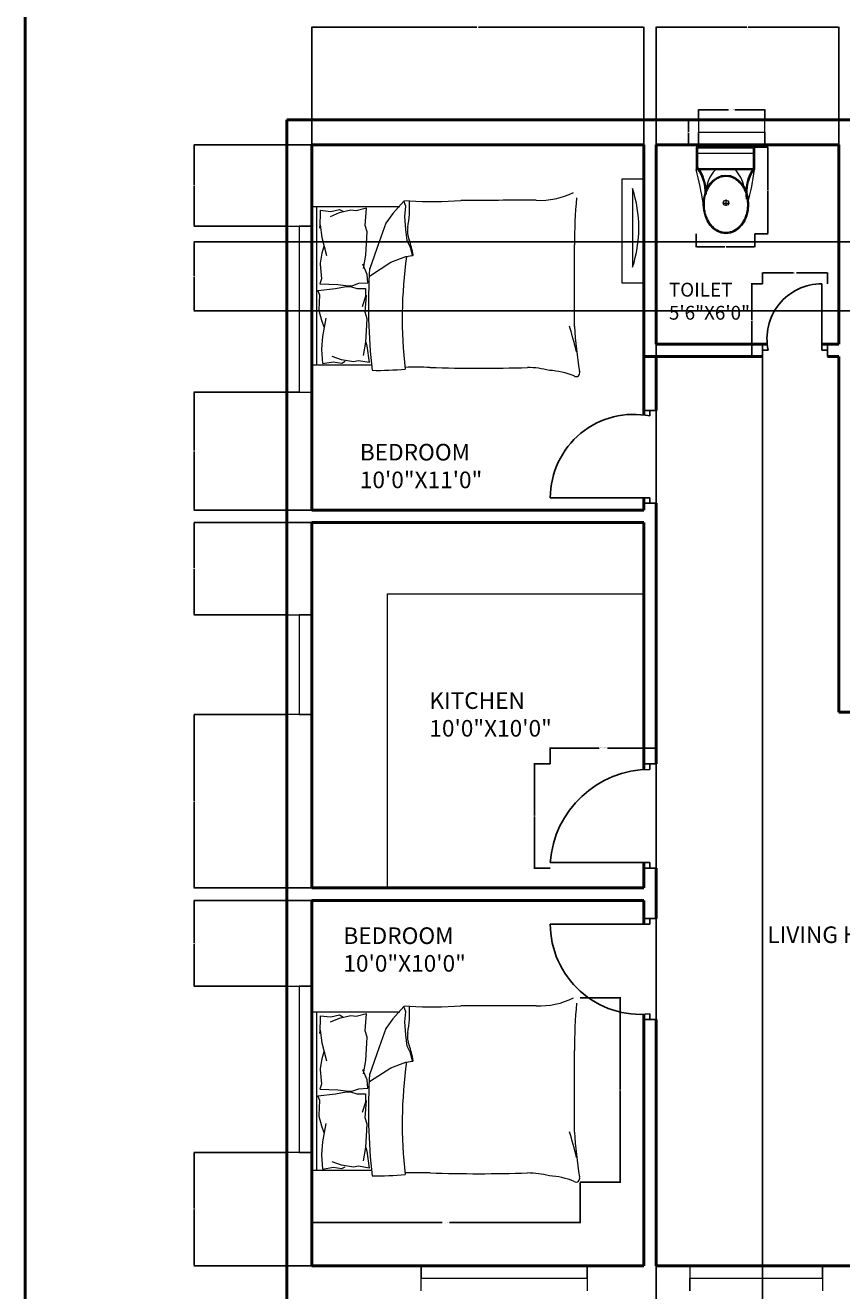
# Model space of a CAD drawing. Units: inches. Extents: x 2268 to 3372, y 1709 to 2892.
# Tile 2 of 6: x 2268 to 2563, y 2040 to 2497. Entities that reach past the tile are written whole.
import ezdxf

# ---------------------------------------------------------------- set-up
doc = ezdxf.new("R2010")
doc.units = ezdxf.units.IN
for name, color, linetype, lineweight in [('A-ANNO-DIMS', 2, 'Continuous', 18), ('A-ANNO-TTLB', 7, 'Continuous', 50), ('A-AREA-IDEN', 7, 'Continuous', 18), ('A-DOOR', 3, 'Continuous', 25), ('A-FLOR-FIXT', 9, 'Continuous', 18), ('A-FURN', 8, 'Continuous', 18), ('A-GLAZ', 4, 'Continuous', 18), ('A-WALL', 7, 'Continuous', 50)]:
    doc.layers.add(name, color=color, linetype=linetype, lineweight=lineweight)
doc.styles.get("Standard").update_dxf_attribs({"font": 'arial.ttf'})
doc.dimstyles.get("Standard").update_dxf_attribs({"dimtxt": 0.18, "dimasz": 0.18, "dimexe": 0.18, "dimexo": 0.0625, "dimgap": 0.09, "dimtad": 0, "dimtih": 1, "dimtoh": 1, "dimdec": 4, "dimzin": 0, "dimdsep": 46, "dimtxsty": 'Standard', "dimcen": 0.09, "dimadec": 0, "dimazin": 0, "dimtfac": 1, "dimtdec": 4, "dimtofl": 0, "dimtmove": 0, "dimatfit": 3, "dimfxl": 1, "dimtolj": 1, "dimtzin": 0, "dimarcsym": 0})

# ---------------------------------------------------------------- blocks, each defined once
blk = doc.blocks.new('A$C31115884')
for p, q in [((283, 498), (223, 498)), ((258, 466), (258, 523)), ((0, 200), (0, 0)), ((520, 200), (0, 200)), ((10, 190), (10, 10)), ((510, 190), (10, 190)), ((510, 10), (510, 190)), ((520, 0), (520, 200)), ((510, 54), (0, 54)), ((10, 10), (510, 10)), ((0, 0), (520, 0))]:
    blk.add_line(p, q)
blk.add_circle((256, 496), 23.6)
for centre, radius, start, end in [((2778, -205), 2807, 165.4549, 171.7133), ((-295, 403), 365, 324.2091, 9.3499), ((-295, 403), 375, 324.2091, 9.3499), ((806, 403), 365, 170.6501, 215.7909), ((3237, 905), 2807, 188.2867, 194.5451), ((384, 406), 293, 190.2774, 224.1564), ((139, 406), 293, 315.8436, 2.6563), ((806, 403), 375, 179.2036, 215.7909)]:
    blk.add_arc(centre, radius, start, end)
blk.add_ellipse((256, 510), major_axis=(0, -261), ratio=0.772727)
blk.add_open_spline([(256, 259), (263, 259), (270, 260), (288, 262), (299, 265), (320, 273), (330, 278), (350, 291), (360, 299), (378, 316), (386, 326), (402, 347), (409, 358), (421, 383), (427, 395), (436, 422), (440, 436), (445, 465), (447, 480), (448, 509), (448, 524), (445, 553), (443, 568), (436, 596), (432, 610), (422, 636), (416, 649), (402, 672), (395, 683), (379, 703), (370, 712), (351, 728), (341, 735), (321, 746), (310, 751), (289, 757), (278, 759), (256, 761), (245, 761), (223, 757), (212, 754), (191, 746), (181, 741), (161, 728), (151, 720), (133, 703), (125, 693), (110, 672), (103, 660), (90, 636), (85, 623), (76, 596), (72, 582), (67, 553), (66, 538), (64, 509), (65, 494), (68, 465), (70, 450), (77, 422), (81, 408), (91, 382), (97, 370), (111, 346), (118, 335), (135, 316), (144, 307), (162, 291), (172, 284), (193, 273), (203, 269), (225, 262), (236, 260), (250, 259), (253, 259), (256, 259)], degree=3, knots=[0, 0, 0, 0, 0.110105, 0.110105, 0.285049, 0.285049, 0.459994, 0.459994, 0.634938, 0.634938, 0.809882, 0.809882, 0.984827, 0.984827, 1.159771, 1.159771, 1.334715, 1.334715, 1.50966, 1.50966, 1.684604, 1.684604, 1.859549, 1.859549, 2.034493, 2.034493, 2.209437, 2.209437, 2.384382, 2.384382, 2.559326, 2.559326, 2.73427, 2.73427, 2.909215, 2.909215, 3.084159, 3.084159, 3.259103, 3.259103, 3.434048, 3.434048, 3.608992, 3.608992, 3.783936, 3.783936, 3.958881, 3.958881, 4.133825, 4.133825, 4.30877, 4.30877, 4.483714, 4.483714, 4.658658, 4.658658, 4.833603, 4.833603, 5.008547, 5.008547, 5.183491, 5.183491, 5.358436, 5.358436, 5.53338, 5.53338, 5.708324, 5.708324, 5.883269, 5.883269, 6.058213, 6.058213, 6.233158, 6.233158, 6.283185, 6.283185, 6.283185, 6.283185])
blk = doc.blocks.new('DOOR-BATH-W')
for p, q in [((21.4, 2.25), (21.4, 26.25)), ((0, 4.5), (0, 0)), ((0, 0), (0, 2.25)), ((0, 2.25), (2, 2.25)), ((23.4, 2.25), (21.4, 2.25)), ((23.4, 4.5), (23.4, 0)), ((23.4, 0), (23.4, 2.25))]:
    blk.add_line(p, q)
blk.add_arc((21.4, 6.41), 19.84, 90, 192.0896)
blk = doc.blocks.new('DOOR-BEDROOM-NW')
for p, q in [((33.75, 33.55), (38.25, 33.55)), ((38.25, 33.55), (36, 33.55)), ((36, 33.55), (36, 31.55)), ((36, 2), (0, 2)), ((33.75, 0), (38.25, 0)), ((36, 0), (36, 2)), ((38.25, 0), (36, 0))]:
    blk.add_line(p, q)
blk.add_arc((30.13, 2), 30.13, 78.7595, 180)
blk = doc.blocks.new('DOOR-BEDROOM-SW')
for p, q in [((36, 34.48), (0, 34.48)), ((33.75, 36.48), (38.25, 36.48)), ((38.25, 36.48), (36, 36.48)), ((36, 36.48), (36, 34.48)), ((33.75, 0), (38.25, 0)), ((36, 0), (36, 2)), ((38.25, 0), (36, 0))]:
    blk.add_line(p, q)
blk.add_arc((32.65, 34.48), 32.65, 180, 275.8823)
blk = doc.blocks.new('DOOR-KITCHEN')
for p, q in [((33.75, 37.66), (38.25, 37.66)), ((38.25, 37.66), (36, 37.66)), ((36, 37.66), (36, 35.66)), ((36, 2), (0, 2)), ((36, 0), (36, 2)), ((33.75, 0), (38.25, 0)), ((38.25, 0), (36, 0))]:
    blk.add_line(p, q)
blk.add_arc((36, -0.42), 36.08, 90, 176.1494)
blk = doc.blocks.new('WIN-48')
for p, q in [((0, 9), (0, 0)), ((48, 4.5), (48, 9)), ((48, 9), (48, 0)), ((0, 0), (0, 4.5)), ((0, 4.5), (48, 4.5))]:
    blk.add_line(p, q)
blk = doc.blocks.new('WIN-60')
for p, q in [((0, 60), (9, 60)), ((9, 60), (4.5, 60)), ((4.5, 60), (4.5, 0)), ((9, 0), (0, 0)), ((4.5, 0), (9, 0))]:
    blk.add_line(p, q)
blk = doc.blocks.new('WIN-60-SPLIT')
for p, q in [((0, 60), (9, 60)), ((9, 60), (4.5, 60)), ((4.5, 60), (4.5, 12)), ((4.5, 12), (4.5, 0)), ((4.5, 0), (0, 0)), ((0, 0), (9, 0))]:
    blk.add_line(p, q)
blk = doc.blocks.new('WIN-36')
for p, q in [((0, 36), (9, 36)), ((9, 36), (4.5, 36)), ((4.5, 36), (4.5, 0)), ((9, 0), (0, 0)), ((4.5, 0), (9, 0))]:
    blk.add_line(p, q)
blk = doc.blocks.new('WIN-24-TRANSVERSE')
for p, q in [((0, 9), (0, 0)), ((24, 0), (24, 9)), ((0, 0), (0, 4.5)), ((0, 4.5), (24, 4.5)), ((24, 4.5), (24, 0))]:
    blk.add_line(p, q)
blk = doc.blocks.new('COUNTER-KITCHEN-L')
for p, q in [((0, 0), (0, 106.22)), ((0, 106.22), (92.56, 106.22))]:
    blk.add_line(p, q)
blk = doc.blocks.new('BEDROOM-WALL-UNIT')
blk.add_line((3.85, 34.02), (3.85, 5.6))
blk.add_lwpolyline([(7.87, 37.37), (0, 37.37), (0, 0), (7.87, 0)], close=True)
blk.add_arc((-39.98, 19.81), 46.08, 342.0375, 17.9625)
blk = doc.blocks.new('BED-DOUBLE')
for p, q in [((0, 61.46), (31.9, 61.46)), ((0, 4.17), (0, 61.46)), ((1.84, 4.17), (1.84, 61.46)), ((3.07, 60.08), (2.95, 53.6)), ((3.07, 60.08), (6.92, 59.62)), ((6.92, 59.62), (10, 60.34)), ((14.18, 60.08), (9.9, 59.11)), ((10, 60.34), (11.25, 59.72)), ((16.11, 59.85), (14.18, 60.08)), ((19.87, 60.78), (16.11, 59.85)), ((19.38, 54.63), (19.87, 60.78)), ((33.26, 63.38), (29.37, 58.94)), ((35.36, 63.48), (33.26, 63.38, 4.64)), ((34.01, 61.54), (33.26, 63.38)), ((33.63, 57.82), (34.01, 61.54)), ((9.9, 59.11), (6.69, 57.7)), ((26.77, 55.41), (24.36, 48.73)), ((29.37, 58.94), (26.77, 55.41)), ((34.01, 53.18), (33.63, 57.82)), ((2.95, 53.6), (3.05, 54.8)), ((3.05, 54.8), (3.68, 50.25)), ((20.05, 52.28), (19.38, 54.63)), ((19.54, 43.87), (20.05, 52.28)), ((34.56, 49.1), (34.01, 53.18)), ((3.68, 50.25), (5.3, 43.75)), ((4.4, 47), (3.69, 44.52)), ((24.36, 48.73), (20.84, 38.73)), ((35.68, 46.68), (34.56, 49.1)), ((36.42, 43.71), (35.68, 46.68)), ((95, 18.06), (95, 47.57)), ((3.69, 44.52), (3.04, 41.01)), ((18.74, 39.04), (19.54, 43.87)), ((20.84, 36.28), (28.62, 41.3)), ((28.62, 41.3), (34.01, 43.34)), ((34.01, 43.34), (36.42, 43.71)), ((3.04, 41.01), (3.07, 40.62)), ((3.07, 40.62), (3.57, 35.31)), ((20.07, 36.86), (18.53, 40.55)), ((20.25, 33.92), (20.07, 36.86)), ((3.57, 35.31), (2.99, 33.54)), ((2.99, 33.54), (9.43, 33.25)), ((8.66, 31.84), (12.47, 32.54)), ((9.43, 33.25), (13.28, 32.79)), ((12.47, 32.54), (14.03, 32.54)), ((13.28, 32.79), (14.84, 32.89)), ((14.03, 32.54), (16.28, 31.84)), ((14.84, 32.89), (17.04, 33.72)), ((17.04, 33.72), (20.25, 33.92)), ((2.24, 31.15), (8.66, 31.84)), ((2.94, 29.42), (2.24, 31.15)), ((2.76, 24.09), (2.94, 29.42)), ((16.28, 31.84), (19.5, 31.84)), ((19.5, 28.9), (18.19, 25.13)), ((19.38, 23.24), (19.87, 29.39)), ((19.5, 31.84), (19.5, 28.9)), ((2.76, 23.7), (2.76, 24.09)), ((3.63, 20.23), (2.76, 23.7)), ((20.05, 20.89), (19.38, 23.24)), ((4.5, 17.81), (3.63, 20.23)), ((3.98, 14.52), (5.19, 21.1)), ((19.54, 12.48), (20.05, 20.89)), ((3.63, 9.93), (3.98, 14.52)), ((3.61, 9.81), (3.63, 9.93)), ((4, 4.67), (3.61, 9.81)), ((18.74, 7.65), (19.54, 12.48)), ((19.54, 12.48), (19.92, 11.13)), ((19.92, 11.13), (20.79, 5.02)), ((3.98, 4.67), (7.79, 5.36)), ((10.74, 6.06), (7.44, 7.27)), ((7.79, 5.36), (10.91, 4.84)), ((15.07, 5.36), (10.74, 6.06)), ((10.91, 4.84), (12.12, 5.54)), ((16.98, 5.71), (15.07, 5.36)), ((20.79, 5.02), (16.98, 5.71)), ((21.71, 4.17), (0, 4.17))]:
    blk.add_line(p, q)
for centre, radius, start, end in [((82.32, 91.3), 27.65, 267.4714, 296.4681), ((254.49, 49.33), 159.5, 174.4998, 180.6351), ((-7.98, 61.53), 43.38, 349.8763, 2.5657), ((43.54, 218.51), 155.25, 266.9791, 273.8365), ((81.31, -5405.34), 5469.02, 90.00217, 90.28689), ((42.04, 52.44), 7.46, 168.6608, 203.7384), ((1.78, 37.35), 35.55, 10.6617, 19.8806), ((187.4, 21.29), 154.68, 171.7845, 186.9006), ((36.49, 43.92), 0.221, 250.2464, 1.1377), ((218.26, 25.61), 197.77, 176.0865, 186.7821), ((-28.43, -20.65), 127.63, 13.3832, 17.7053), ((240.78, 25.69), 145.97, 182.9958, 189.4091), ((24.09, 102.1), 99.87, 268.7218, 275.604), ((37.37, -200.58), 203.94, 88.4762, 91.0082), ((60.68, 581.23), 578.22, 268.22771, 271.71854), ((77.34, -32.25), 35.53, 76.0648, 88.9113), ((84.25, -25.97), 28.25, 67.9751, 86.652), ((95.57, 1.3), 1.31, 236.1736, 23.4781)]:
    blk.add_arc(centre, radius, start, end)
blk = doc.blocks.new('*D34')
at = {"layer": 'A-ANNO-DIMS', "color": 0, "lineweight": -2, "transparency": 16777216}
for p, q in [((2534.82, 2403.93), (2530.76, 2403.93)), ((2530.94, 2403.75), (2530.94, 2390.98)), ((2530.94, 2377.86), (2530.94, 2390.62)), ((2534.82, 2377.68), (2530.76, 2377.68))]:
    blk.add_line(p, q, dxfattribs=at)
at = {"layer": 'A-ANNO-DIMS', "color": 0, "transparency": 16777216}
for points in [[(2530.91, 2403.75), (2530.97, 2403.75), (2530.94, 2403.93)], [(2530.91, 2377.86), (2530.97, 2377.86), (2530.94, 2377.68)]]:
    blk.add_solid(points, dxfattribs=at)
at = {"layer": 'Defpoints', "color": 0, "transparency": 16777216}
for p in [(2530.94, 2403.93), (2534.88, 2403.93), (2534.88, 2377.68)]:
    blk.add_point(p, dxfattribs=at)
at = {"layer": 'A-ANNO-DIMS', "color": 0, "transparency": 16777216, "insert": (2530.94, 2390.8), "char_height": 0.18, "attachment_point": 5}
blk.add_mtext('\\A1;DOOR 26 TYP.', dxfattribs=at)
blk = doc.blocks.new('*D35')
at = {"layer": 'A-ANNO-DIMS', "color": 0, "lineweight": -2, "transparency": 16777216}
for p, q in [((2534.88, 2403.99), (2534.88, 2408.04)), ((2535.06, 2407.86), (2546.05, 2407.86)), ((2558.1, 2407.86), (2547.11, 2407.86)), ((2558.28, 2403.99), (2558.28, 2408.04))]:
    blk.add_line(p, q, dxfattribs=at)
at = {"layer": 'A-ANNO-DIMS', "color": 0, "transparency": 16777216}
for points in [[(2535.06, 2407.89), (2535.06, 2407.83), (2534.88, 2407.86)], [(2558.1, 2407.89), (2558.1, 2407.83), (2558.28, 2407.86)]]:
    blk.add_solid(points, dxfattribs=at)
at = {"layer": 'Defpoints', "color": 0, "transparency": 16777216}
for p in [(2558.28, 2407.86), (2534.88, 2403.93), (2558.28, 2403.93)]:
    blk.add_point(p, dxfattribs=at)
at = {"layer": 'A-ANNO-DIMS', "color": 0, "transparency": 16777216, "insert": (2546.58, 2407.86), "char_height": 0.18, "attachment_point": 5}
blk.add_mtext('\\A1;23 TYP.', dxfattribs=at)
blk = doc.blocks.new('*D42')
at = {"layer": 'A-ANNO-DIMS', "color": 0, "lineweight": -2, "transparency": 16777216}
for p, q in [((2458.14, 2230.55), (2458.14, 2236.4)), ((2458.32, 2236.22), (2475.75, 2236.22)), ((2496.21, 2236.22), (2478.79, 2236.22)), ((2496.39, 2230.55), (2496.39, 2236.4))]:
    blk.add_line(p, q, dxfattribs=at)
at = {"layer": 'A-ANNO-DIMS', "color": 0, "transparency": 16777216}
for points in [[(2458.32, 2236.25), (2458.32, 2236.19), (2458.14, 2236.22)], [(2496.21, 2236.25), (2496.21, 2236.19), (2496.39, 2236.22)]]:
    blk.add_solid(points, dxfattribs=at)
at = {"layer": 'Defpoints', "color": 0, "transparency": 16777216}
for p in [(2496.39, 2236.22), (2458.14, 2230.49), (2496.39, 2230.49)]:
    blk.add_point(p, dxfattribs=at)
at = {"layer": 'A-ANNO-DIMS', "color": 0, "transparency": 16777216, "insert": (2477.27, 2236.22), "char_height": 0.18, "attachment_point": 5}
blk.add_mtext('\\A1;KITCHEN DOOR 38 TYP.', dxfattribs=at)
blk = doc.blocks.new('*D43')
at = {"layer": 'A-ANNO-DIMS', "color": 0, "lineweight": -2, "transparency": 16777216}
for p, q in [((2458.08, 2230.49), (2452.23, 2230.49)), ((2452.41, 2230.31), (2452.41, 2211.84)), ((2452.41, 2193.01), (2452.41, 2211.47)), ((2458.08, 2192.83), (2452.23, 2192.83))]:
    blk.add_line(p, q, dxfattribs=at)
at = {"layer": 'A-ANNO-DIMS', "color": 0, "transparency": 16777216}
for points in [[(2452.38, 2230.31), (2452.44, 2230.31), (2452.41, 2230.49)], [(2452.38, 2193.01), (2452.44, 2193.01), (2452.41, 2192.83)]]:
    blk.add_solid(points, dxfattribs=at)
at = {"layer": 'Defpoints', "color": 0, "transparency": 16777216}
for p in [(2452.41, 2230.49), (2458.14, 2230.49), (2458.14, 2192.83)]:
    blk.add_point(p, dxfattribs=at)
at = {"layer": 'A-ANNO-DIMS', "color": 0, "transparency": 16777216, "insert": (2452.41, 2211.66), "char_height": 0.18, "attachment_point": 5}
blk.add_mtext('\\A1;38 TYP.', dxfattribs=at)
blk = doc.blocks.new('*D48')
at = {"layer": 'A-ANNO-DIMS', "color": 0, "lineweight": -2, "transparency": 16777216}
for p, q in [((2511.69, 2463.24), (2511.69, 2466.96)), ((2511.87, 2466.78), (2522.57, 2466.78)), ((2535.51, 2466.78), (2524.81, 2466.78)), ((2535.69, 2463.24), (2535.69, 2466.96))]:
    blk.add_line(p, q, dxfattribs=at)
at = {"layer": 'A-ANNO-DIMS', "color": 0, "transparency": 16777216}
for points in [[(2511.87, 2466.81), (2511.87, 2466.75), (2511.69, 2466.78)], [(2535.51, 2466.81), (2535.51, 2466.75), (2535.69, 2466.78)]]:
    blk.add_solid(points, dxfattribs=at)
at = {"layer": 'Defpoints', "color": 0, "transparency": 16777216}
for p in [(2535.69, 2466.78), (2511.69, 2463.18), (2535.69, 2463.18)]:
    blk.add_point(p, dxfattribs=at)
at = {"layer": 'A-ANNO-DIMS', "color": 0, "transparency": 16777216, "insert": (2523.69, 2466.78), "char_height": 0.18, "attachment_point": 5}
blk.add_mtext('\\A1;WINDOW 24 TYP.', dxfattribs=at)
blk = doc.blocks.new('*D49')
at = {"layer": 'A-ANNO-DIMS', "color": 0, "lineweight": -2, "transparency": 16777216}
for p, q in [((2511.63, 2463.18), (2507.91, 2463.18)), ((2508.09, 2463), (2508.09, 2458.86)), ((2508.09, 2454.36), (2508.09, 2458.49)), ((2511.63, 2454.18), (2507.91, 2454.18))]:
    blk.add_line(p, q, dxfattribs=at)
at = {"layer": 'A-ANNO-DIMS', "color": 0, "transparency": 16777216}
for points in [[(2508.06, 2463), (2508.12, 2463), (2508.09, 2463.18)], [(2508.06, 2454.36), (2508.12, 2454.36), (2508.09, 2454.18)]]:
    blk.add_solid(points, dxfattribs=at)
at = {"layer": 'Defpoints', "color": 0, "transparency": 16777216}
for p in [(2508.09, 2463.18), (2511.69, 2463.18), (2511.69, 2454.18)]:
    blk.add_point(p, dxfattribs=at)
at = {"layer": 'A-ANNO-DIMS', "color": 0, "transparency": 16777216, "insert": (2508.09, 2458.68), "char_height": 0.18, "attachment_point": 5}
blk.add_mtext('\\A1;9 TYP.', dxfattribs=at)
blk = doc.blocks.new('*D70')
at = {"layer": 'A-ANNO-DIMS', "color": 0, "lineweight": -2, "transparency": 16777216}
for p, q in [((2371.89, 2079.27), (2371.89, 2064.61)), ((2468.89, 2079.27), (2468.89, 2064.61)), ((2372.07, 2064.79), (2419.02, 2064.79)), ((2468.71, 2064.79), (2421.76, 2064.79))]:
    blk.add_line(p, q, dxfattribs=at)
at = {"layer": 'A-ANNO-DIMS', "color": 0, "transparency": 16777216}
for points in [[(2372.07, 2064.82), (2372.07, 2064.76), (2371.89, 2064.79)], [(2468.71, 2064.82), (2468.71, 2064.76), (2468.89, 2064.79)]]:
    blk.add_solid(points, dxfattribs=at)
at = {"layer": 'Defpoints', "color": 0, "transparency": 16777216}
for p in [(2371.89, 2079.34), (2468.89, 2079.34), (2468.89, 2064.79)]:
    blk.add_point(p, dxfattribs=at)
at = {"layer": 'A-ANNO-DIMS', "color": 0, "transparency": 16777216, "insert": (2420.39, 2064.79), "char_height": 0.18, "attachment_point": 5}
blk.add_mtext('\\A1;DOUBLE BED 97 TYP.', dxfattribs=at)
blk = doc.blocks.new('*D71')
at = {"layer": 'A-ANNO-DIMS', "color": 0, "lineweight": -2, "transparency": 16777216}
for p, q in [((2468.96, 2145.99), (2483.62, 2145.99)), ((2483.44, 2145.81), (2483.44, 2112.84)), ((2483.44, 2079.52), (2483.44, 2112.48)), ((2468.96, 2079.34), (2483.62, 2079.34))]:
    blk.add_line(p, q, dxfattribs=at)
at = {"layer": 'A-ANNO-DIMS', "color": 0, "transparency": 16777216}
for points in [[(2483.41, 2145.81), (2483.47, 2145.81), (2483.44, 2145.99)], [(2483.41, 2079.52), (2483.47, 2079.52), (2483.44, 2079.34)]]:
    blk.add_solid(points, dxfattribs=at)
at = {"layer": 'Defpoints', "color": 0, "transparency": 16777216}
for p in [(2468.89, 2145.99), (2483.44, 2145.99), (2468.89, 2079.34)]:
    blk.add_point(p, dxfattribs=at)
at = {"layer": 'A-ANNO-DIMS', "color": 0, "transparency": 16777216, "insert": (2483.44, 2112.66), "char_height": 0.18, "attachment_point": 5}
blk.add_mtext('\\A1;67 TYP.', dxfattribs=at)
blk = doc.blocks.new('*D74')
at = {"layer": 'A-ANNO-DIMS', "color": 0, "lineweight": -2, "transparency": 16777216}
for p, q in [((2532.07, 2453.35), (2536.88, 2453.35)), ((2536.7, 2453.17), (2536.7, 2437.88)), ((2536.7, 2422.22), (2536.7, 2437.51)), ((2532.07, 2422.04), (2536.88, 2422.04))]:
    blk.add_line(p, q, dxfattribs=at)
at = {"layer": 'A-ANNO-DIMS', "color": 0, "transparency": 16777216}
for points in [[(2536.67, 2453.17), (2536.73, 2453.17), (2536.7, 2453.35)], [(2536.67, 2422.22), (2536.73, 2422.22), (2536.7, 2422.04)]]:
    blk.add_solid(points, dxfattribs=at)
at = {"layer": 'Defpoints', "color": 0, "transparency": 16777216}
for p in [(2532, 2453.35), (2532, 2422.04), (2536.7, 2422.04)]:
    blk.add_point(p, dxfattribs=at)
at = {"layer": 'A-ANNO-DIMS', "color": 0, "transparency": 16777216, "insert": (2536.7, 2437.7), "char_height": 0.18, "attachment_point": 5}
blk.add_mtext('\\A1;WC 31', dxfattribs=at)
blk = doc.blocks.new('*D75')
at = {"layer": 'A-ANNO-DIMS', "color": 0, "lineweight": -2, "transparency": 16777216}
for p, q in [((2510.88, 2421.98), (2510.88, 2417.17)), ((2532, 2421.98), (2532, 2417.17)), ((2511.06, 2417.35), (2521.24, 2417.35)), ((2531.82, 2417.35), (2521.65, 2417.35))]:
    blk.add_line(p, q, dxfattribs=at)
at = {"layer": 'A-ANNO-DIMS', "color": 0, "transparency": 16777216}
for points in [[(2511.06, 2417.38), (2511.06, 2417.32), (2510.88, 2417.35)], [(2531.82, 2417.38), (2531.82, 2417.32), (2532, 2417.35)]]:
    blk.add_solid(points, dxfattribs=at)
at = {"layer": 'Defpoints', "color": 0, "transparency": 16777216}
for p in [(2510.88, 2422.04), (2532, 2422.04), (2510.88, 2417.35)]:
    blk.add_point(p, dxfattribs=at)
at = {"layer": 'A-ANNO-DIMS', "color": 0, "transparency": 16777216, "insert": (2521.44, 2417.35), "char_height": 0.18, "attachment_point": 5}
blk.add_mtext('\\A1;21', dxfattribs=at)
blk = doc.blocks.new('*D78')
at = {"layer": 'A-ANNO-DIMS', "color": 0, "lineweight": -2, "transparency": 16777216}
for p, q in [((2371.89, 2454.24), (2371.89, 2496.81)), ((2372.07, 2496.63), (2431.61, 2496.63)), ((2491.71, 2496.63), (2432.17, 2496.63)), ((2491.89, 2454.24), (2491.89, 2496.81))]:
    blk.add_line(p, q, dxfattribs=at)
at = {"layer": 'A-ANNO-DIMS', "color": 0, "transparency": 16777216}
for points in [[(2372.07, 2496.66), (2372.07, 2496.6), (2371.89, 2496.63)], [(2491.71, 2496.66), (2491.71, 2496.6), (2491.89, 2496.63)]]:
    blk.add_solid(points, dxfattribs=at)
at = {"layer": 'Defpoints', "color": 0, "transparency": 16777216}
for p in [(2491.89, 2496.63), (2371.89, 2454.18), (2491.89, 2454.18)]:
    blk.add_point(p, dxfattribs=at)
at = {"layer": 'A-ANNO-DIMS', "color": 0, "transparency": 16777216, "insert": (2431.89, 2496.63), "char_height": 0.18, "attachment_point": 5}
blk.add_mtext('\\A1;120', dxfattribs=at)
blk = doc.blocks.new('*D79')
at = {"layer": 'A-ANNO-DIMS', "color": 0, "lineweight": -2, "transparency": 16777216}
for p, q in [((2496.39, 2454.24), (2496.39, 2496.81)), ((2496.57, 2496.63), (2529.17, 2496.63)), ((2562.21, 2496.63), (2529.61, 2496.63)), ((2562.39, 2454.24), (2562.39, 2496.81))]:
    blk.add_line(p, q, dxfattribs=at)
at = {"layer": 'A-ANNO-DIMS', "color": 0, "transparency": 16777216}
for points in [[(2496.57, 2496.66), (2496.57, 2496.6), (2496.39, 2496.63)], [(2562.21, 2496.66), (2562.21, 2496.6), (2562.39, 2496.63)]]:
    blk.add_solid(points, dxfattribs=at)
at = {"layer": 'Defpoints', "color": 0, "transparency": 16777216}
for p in [(2562.39, 2496.63), (2496.39, 2454.18), (2562.39, 2454.18)]:
    blk.add_point(p, dxfattribs=at)
at = {"layer": 'A-ANNO-DIMS', "color": 0, "transparency": 16777216, "insert": (2529.39, 2496.63), "char_height": 0.18, "attachment_point": 5}
blk.add_mtext('\\A1;66', dxfattribs=at)
blk = doc.blocks.new('*D81')
at = {"layer": 'A-ANNO-DIMS', "color": 0, "lineweight": -2, "transparency": 16777216}
for p, q in [((2496.39, 2382.11), (2496.39, 1790.27)), ((2534.88, 2377.61), (2534.88, 1790.27)), ((2496.57, 1790.45), (2515.17, 1790.45)), ((2534.7, 1790.45), (2516.1, 1790.45))]:
    blk.add_line(p, q, dxfattribs=at)
at = {"layer": 'A-ANNO-DIMS', "color": 0, "transparency": 16777216}
for points in [[(2496.57, 1790.48), (2496.57, 1790.42), (2496.39, 1790.45)], [(2534.7, 1790.48), (2534.7, 1790.42), (2534.88, 1790.45)]]:
    blk.add_solid(points, dxfattribs=at)
at = {"layer": 'Defpoints', "color": 0, "transparency": 16777216}
for p in [(2496.39, 2382.18), (2534.88, 2377.68), (2534.88, 1790.45)]:
    blk.add_point(p, dxfattribs=at)
at = {"layer": 'A-ANNO-DIMS', "color": 0, "transparency": 16777216, "insert": (2515.64, 1790.45), "char_height": 0.18, "attachment_point": 5}
blk.add_mtext('\\A1;38.486', dxfattribs=at)
blk = doc.blocks.new('*D84')
at = {"layer": 'A-ANNO-DIMS', "color": 0, "lineweight": -2, "transparency": 16777216}
for p, q in [((2362.83, 2090.16), (2329.26, 2090.16)), ((2329.44, 2089.98), (2329.44, 2069.85)), ((2329.44, 2049.36), (2329.44, 2069.49)), ((2371.83, 2049.18), (2329.26, 2049.18))]:
    blk.add_line(p, q, dxfattribs=at)
at = {"layer": 'A-ANNO-DIMS', "color": 0, "transparency": 16777216}
for points in [[(2329.41, 2089.98), (2329.47, 2089.98), (2329.44, 2090.16)], [(2329.41, 2049.36), (2329.47, 2049.36), (2329.44, 2049.18)]]:
    blk.add_solid(points, dxfattribs=at)
at = {"layer": 'Defpoints', "color": 0, "transparency": 16777216}
for p in [(2329.44, 2090.16), (2362.89, 2090.16), (2371.89, 2049.18)]:
    blk.add_point(p, dxfattribs=at)
at = {"layer": 'A-ANNO-DIMS', "color": 0, "transparency": 16777216, "insert": (2329.44, 2069.67), "char_height": 0.18, "attachment_point": 5}
blk.add_mtext('\\A1;40.986', dxfattribs=at)
blk = doc.blocks.new('*D85')
at = {"layer": 'A-ANNO-DIMS', "color": 0, "lineweight": -2, "transparency": 16777216}
for p, q in [((2371.83, 2181.18), (2329.26, 2181.18)), ((2329.44, 2181), (2329.44, 2165.85)), ((2329.44, 2150.34), (2329.44, 2165.49)), ((2362.83, 2150.16), (2329.26, 2150.16))]:
    blk.add_line(p, q, dxfattribs=at)
at = {"layer": 'A-ANNO-DIMS', "color": 0, "transparency": 16777216}
for points in [[(2329.41, 2181), (2329.47, 2181), (2329.44, 2181.18)], [(2329.41, 2150.34), (2329.47, 2150.34), (2329.44, 2150.16)]]:
    blk.add_solid(points, dxfattribs=at)
at = {"layer": 'Defpoints', "color": 0, "transparency": 16777216}
for p in [(2329.44, 2181.18), (2371.89, 2181.18), (2362.89, 2150.16)]:
    blk.add_point(p, dxfattribs=at)
at = {"layer": 'A-ANNO-DIMS', "color": 0, "transparency": 16777216, "insert": (2329.44, 2165.67), "char_height": 0.18, "attachment_point": 5}
blk.add_mtext('\\A1;31.014', dxfattribs=at)
blk = doc.blocks.new('*D86')
at = {"layer": 'A-ANNO-DIMS', "color": 0, "lineweight": -2, "transparency": 16777216}
for p, q in [((2362.83, 2248.31), (2329.26, 2248.31)), ((2329.44, 2248.13), (2329.44, 2217.17)), ((2329.44, 2185.86), (2329.44, 2216.81)), ((2371.83, 2185.68), (2329.26, 2185.68))]:
    blk.add_line(p, q, dxfattribs=at)
at = {"layer": 'A-ANNO-DIMS', "color": 0, "transparency": 16777216}
for points in [[(2329.41, 2248.13), (2329.47, 2248.13), (2329.44, 2248.31)], [(2329.41, 2185.86), (2329.47, 2185.86), (2329.44, 2185.68)]]:
    blk.add_solid(points, dxfattribs=at)
at = {"layer": 'Defpoints', "color": 0, "transparency": 16777216}
for p in [(2329.44, 2248.31), (2362.89, 2248.31), (2371.89, 2185.68)]:
    blk.add_point(p, dxfattribs=at)
at = {"layer": 'A-ANNO-DIMS', "color": 0, "transparency": 16777216, "insert": (2329.44, 2216.99), "char_height": 0.18, "attachment_point": 5}
blk.add_mtext('\\A1;62.63', dxfattribs=at)
blk = doc.blocks.new('*D87')
at = {"layer": 'A-ANNO-DIMS', "color": 0, "lineweight": -2, "transparency": 16777216}
for p, q in [((2371.83, 2317.68), (2329.26, 2317.68)), ((2329.44, 2317.5), (2329.44, 2301.17)), ((2329.44, 2284.49), (2329.44, 2300.81)), ((2362.83, 2284.31), (2329.26, 2284.31))]:
    blk.add_line(p, q, dxfattribs=at)
at = {"layer": 'A-ANNO-DIMS', "color": 0, "transparency": 16777216}
for points in [[(2329.41, 2317.5), (2329.47, 2317.5), (2329.44, 2317.68)], [(2329.41, 2284.49), (2329.47, 2284.49), (2329.44, 2284.31)]]:
    blk.add_solid(points, dxfattribs=at)
at = {"layer": 'Defpoints', "color": 0, "transparency": 16777216}
for p in [(2329.44, 2317.68), (2371.89, 2317.68), (2362.89, 2284.31)]:
    blk.add_point(p, dxfattribs=at)
at = {"layer": 'A-ANNO-DIMS', "color": 0, "transparency": 16777216, "insert": (2329.44, 2300.99), "char_height": 0.18, "attachment_point": 5}
blk.add_mtext('\\A1;33.37', dxfattribs=at)
blk = doc.blocks.new('*D88')
at = {"layer": 'A-ANNO-DIMS', "color": 0, "lineweight": -2, "transparency": 16777216}
for p, q in [((2362.83, 2364.81), (2329.26, 2364.81)), ((2329.44, 2364.63), (2329.44, 2343.68)), ((2329.44, 2322.36), (2329.44, 2343.31)), ((2371.83, 2322.18), (2329.26, 2322.18))]:
    blk.add_line(p, q, dxfattribs=at)
at = {"layer": 'A-ANNO-DIMS', "color": 0, "transparency": 16777216}
for points in [[(2329.41, 2364.63), (2329.47, 2364.63), (2329.44, 2364.81)], [(2329.41, 2322.36), (2329.47, 2322.36), (2329.44, 2322.18)]]:
    blk.add_solid(points, dxfattribs=at)
at = {"layer": 'Defpoints', "color": 0, "transparency": 16777216}
for p in [(2329.44, 2364.81), (2362.89, 2364.81), (2371.89, 2322.18)]:
    blk.add_point(p, dxfattribs=at)
at = {"layer": 'A-ANNO-DIMS', "color": 0, "transparency": 16777216, "insert": (2329.44, 2343.49), "char_height": 0.18, "attachment_point": 5}
blk.add_mtext('\\A1;42.64', dxfattribs=at)
blk = doc.blocks.new('*D89')
at = {"layer": 'A-ANNO-DIMS', "color": 0, "lineweight": -2, "transparency": 16777216}
for p, q in [((2371.83, 2454.18), (2329.26, 2454.18)), ((2329.44, 2454), (2329.44, 2439.68)), ((2329.44, 2424.99), (2329.44, 2439.31)), ((2362.83, 2424.81), (2329.26, 2424.81))]:
    blk.add_line(p, q, dxfattribs=at)
at = {"layer": 'A-ANNO-DIMS', "color": 0, "transparency": 16777216}
for points in [[(2329.41, 2454), (2329.47, 2454), (2329.44, 2454.18)], [(2329.41, 2424.99), (2329.47, 2424.99), (2329.44, 2424.81)]]:
    blk.add_solid(points, dxfattribs=at)
at = {"layer": 'Defpoints', "color": 0, "transparency": 16777216}
for p in [(2329.44, 2454.18), (2371.89, 2454.18), (2362.89, 2424.81)]:
    blk.add_point(p, dxfattribs=at)
at = {"layer": 'A-ANNO-DIMS', "color": 0, "transparency": 16777216, "insert": (2329.44, 2439.49), "char_height": 0.18, "attachment_point": 5}
blk.add_mtext('\\A1;29.36', dxfattribs=at)
blk = doc.blocks.new('*D98')
at = {"layer": 'A-ANNO-DIMS', "color": 0, "lineweight": -2, "transparency": 16777216}
for p, q in [((2703.83, 2419.05), (2329.26, 2419.05)), ((2329.44, 2418.87), (2329.44, 2406.8)), ((2329.44, 2394.36), (2329.44, 2406.43)), ((2703.83, 2394.18), (2329.26, 2394.18))]:
    blk.add_line(p, q, dxfattribs=at)
at = {"layer": 'A-ANNO-DIMS', "color": 0, "transparency": 16777216}
for points in [[(2329.41, 2418.87), (2329.47, 2418.87), (2329.44, 2419.05)], [(2329.41, 2394.36), (2329.47, 2394.36), (2329.44, 2394.18)]]:
    blk.add_solid(points, dxfattribs=at)
at = {"layer": 'Defpoints', "color": 0, "transparency": 16777216}
for p in [(2329.44, 2419.05), (2703.89, 2419.05), (2703.89, 2394.18)]:
    blk.add_point(p, dxfattribs=at)
at = {"layer": 'A-ANNO-DIMS', "color": 0, "transparency": 16777216, "insert": (2329.44, 2406.61), "char_height": 0.18, "attachment_point": 5}
blk.add_mtext('\\A1;24.88', dxfattribs=at)

msp = doc.modelspace()

# ---------------------------------------------------------------- linework, layer by layer
at = {"layer": 'A-ANNO-TTLB'}
msp.add_lwpolyline([(2268.3884, 2892.2471), (3372.3464, 2892.2471), (3372.3464, 1709.0755), (2268.3884, 1709.0755)], close=True, dxfattribs=at)
at = {"layer": 'A-WALL'}
for p, q in [((2362.8943, 2463.1756), (2712.8943, 2463.1756)), ((2362.8943, 2463.1756), (2712.8943, 2463.1756)), ((2362.8943, 2463.1756), (2362.8943, 1877.1756)), ((2362.8943, 2463.1756), (2712.8943, 2463.1756)), ((2362.8943, 2463.1756), (2712.8943, 2463.1756)), ((2362.8943, 2463.1756), (2362.8943, 1877.1756)), ((2371.8943, 2454.1756), (2491.8943, 2454.1756)), ((2371.8943, 2454.1756), (2371.8943, 2322.1756)), ((2371.8943, 2454.1756), (2491.8943, 2454.1756)), ((2371.8943, 2454.1756), (2371.8943, 2322.1756)), ((2491.8943, 2454.1756), (2491.8943, 2356.5449)), ((2491.8943, 2454.1756), (2491.8943, 2356.5449)), ((2496.3943, 2454.1756), (2496.3943, 2382.1756)), ((2496.3943, 2454.1756), (2562.3943, 2454.1756)), ((2496.3943, 2454.1756), (2562.3943, 2454.1756)), ((2496.3943, 2454.1756), (2496.3943, 2382.1756)), ((2562.3943, 2454.1756), (2562.3943, 2382.1756)), ((2562.3943, 2454.1756), (2562.3943, 2382.1756)), ((2496.3943, 2382.1756), (2536.5315, 2382.1756)), ((2496.3943, 2382.1756), (2536.5315, 2382.1756)), ((2556.2836, 2382.1756), (2562.3943, 2382.1756)), ((2556.2836, 2382.1756), (2562.3943, 2382.1756)), ((2491.8943, 2377.6756), (2534.8799, 2377.6756)), ((2491.8943, 2377.6756), (2534.8799, 2377.6756)), ((2496.3943, 2377.6756), (2496.3943, 2358.1856)), ((2496.3943, 2377.6756), (2496.3943, 2358.1856)), ((2558.2836, 2377.6756), (2562.3943, 2377.6756)), ((2558.2836, 2377.6756), (2562.3943, 2377.6756)), ((2562.3943, 2377.6756), (2562.3943, 2249.1756)), ((2562.3943, 2377.6756), (2562.3943, 2249.1756)), ((2491.8943, 2326.6361), (2491.8943, 2322.1756)), ((2491.8943, 2326.6361), (2491.8943, 2322.1756)), ((2496.3943, 2324.6361), (2496.3943, 2230.4862)), ((2496.3943, 2324.6361), (2496.3943, 2230.4862)), ((2371.8943, 2322.1756), (2491.8943, 2322.1756)), ((2371.8943, 2322.1756), (2491.8943, 2322.1756)), ((2371.8943, 2317.6756), (2491.8943, 2317.6756)), ((2371.8943, 2317.6756), (2371.8943, 2185.6756)), ((2371.8943, 2317.6756), (2491.8943, 2317.6756)), ((2371.8943, 2317.6756), (2371.8943, 2185.6756)), ((2491.8943, 2317.6756), (2491.8943, 2228.4159)), ((2491.8943, 2317.6756), (2491.8943, 2228.4159)), ((2566.8943, 2249.1756), (2562.3943, 2249.1756)), ((2566.8943, 2249.1756), (2562.3943, 2249.1756)), ((2491.8943, 2194.8278), (2491.8943, 2185.6756)), ((2491.8943, 2194.8278), (2491.8943, 2185.6756)), ((2496.3943, 2192.8278), (2496.3943, 2174.6517)), ((2496.3943, 2192.8278), (2496.3943, 2174.6517)), ((2371.8943, 2185.6756), (2491.8943, 2185.6756)), ((2371.8943, 2185.6756), (2491.8943, 2185.6756)), ((2371.8943, 2181.1756), (2491.8943, 2181.1756)), ((2371.8943, 2181.1756), (2371.8943, 2049.1756)), ((2371.8943, 2181.1756), (2491.8943, 2181.1756)), ((2371.8943, 2181.1756), (2371.8943, 2049.1756)), ((2491.8943, 2181.1756), (2491.8943, 2172.6517)), ((2491.8943, 2181.1756), (2491.8943, 2172.6517)), ((2491.8943, 2140.0166), (2491.8943, 2049.1756)), ((2491.8943, 2140.0166), (2491.8943, 2049.1756)), ((2496.3943, 2138.1701), (2496.3943, 2049.1756)), ((2496.3943, 2138.1701), (2496.3943, 2049.1756)), ((2371.8943, 2049.1756), (2491.8943, 2049.1756)), ((2371.8943, 2049.1756), (2491.8943, 2049.1756)), ((2496.3943, 2049.1756), (2571.2467, 2049.1756)), ((2496.3943, 2049.1756), (2571.2467, 2049.1756))]:
    msp.add_line(p, q, dxfattribs=at)

# ---------------------------------------------------------------- block references
at = {"layer": 'A-DOOR'}
for name, p in [('DOOR-BATH-W', (2534.88, 2377.676)), ('DOOR-BATH-W', (2534.88, 2377.676)), ('DOOR-BEDROOM-NW', (2458.144, 2324.636)), ('DOOR-BEDROOM-NW', (2458.144, 2324.636)), ('DOOR-KITCHEN', (2458.144, 2192.828)), ('DOOR-KITCHEN', (2458.144, 2192.828)), ('DOOR-BEDROOM-SW', (2458.144, 2138.17)), ('DOOR-BEDROOM-SW', (2458.144, 2138.17))]:
    msp.add_blockref(name, p, dxfattribs=at)
at = {"layer": 'A-FLOR-FIXT', "xscale": 0.0406268506401408, "yscale": 0.0406268506401408, "zscale": 0.0406268506401408, "rotation": 179.9999999999998}
msp.add_blockref('A$C31115884', (2532.0049, 2453.3491), dxfattribs=at)
at = {"layer": 'A-FLOR-FIXT'}
msp.add_blockref('COUNTER-KITCHEN-L', (2399.33, 2185.676), dxfattribs=at)
msp.add_blockref('COUNTER-KITCHEN-L', (2399.33, 2185.676), dxfattribs=at)
at = {"layer": 'A-FURN'}
for name, p in [('BEDROOM-WALL-UNIT', (2484.029, 2404.345)), ('BEDROOM-WALL-UNIT', (2484.029, 2404.345)), ('BED-DOUBLE', (2371.894, 2370.4326)), ('BED-DOUBLE', (2371.894, 2079.439))]:
    msp.add_blockref(name, p, dxfattribs=at)
at = {"layer": 'A-GLAZ'}
for name, p in [('WIN-24-TRANSVERSE', (2511.69, 2454.176)), ('WIN-24-TRANSVERSE', (2511.69, 2454.176)), ('WIN-60-SPLIT', (2362.894, 2364.813)), ('WIN-60-SPLIT', (2362.894, 2364.813)), ('WIN-36', (2362.894, 2248.308)), ('WIN-36', (2362.894, 2248.308)), ('WIN-60', (2362.894, 2090.161)), ('WIN-60', (2362.894, 2090.161)), ('WIN-48', (2508.522, 2040.176)), ('WIN-48', (2508.522, 2040.176))]:
    msp.add_blockref(name, p, dxfattribs=at)
for rotation in [89.99999999999905, 89.9999999999979]:
    msp.add_blockref('WIN-60', (2471.4241, 2040.1753), dxfattribs=dict(at, rotation=rotation))

# ---------------------------------------------------------------- texts
at = {"layer": 'A-AREA-IDEN', "attachment_point": 1}
for s, width, insert, char_height in [('TOILET\\P5\'6"X6\'0"', 92.018974, (2501.0105, 2404.318), 5), ('TOILET\\P5\'6"X6\'0"', 92.018974, (2501.0105, 2404.318), 5), ('BEDROOM\\P10\'0"X11\'0"', 158.479811, (2389.2994, 2346.1068), 6), ('BEDROOM\\P10\'0"X11\'0"', 158.479811, (2389.2994, 2346.1068), 6), ('KITCHEN\\P10\'0"X10\'0"', 100.075673, (2414.4311, 2256.3609), 6), ('KITCHEN\\P10\'0"X10\'0"', 100.075673, (2414.4311, 2256.3609), 6), ('BEDROOM\\P10\'0"X10\'0"', 136.415087, (2383.3623, 2171.4295), 6), ('BEDROOM\\P10\'0"X10\'0"', 136.415087, (2383.3623, 2171.4295), 6), ('LIVING HALL', 226.155765, (2536.5837, 2171.7788), 6)]:
    msp.add_mtext_dynamic_manual_height_columns(s, width=width, gutter_width=12.5, heights=[0], dxfattribs=dict(at, insert=insert, char_height=char_height))

# ---------------------------------------------------------------- dimensions: what is measured, and where the dimension line sits
at = {"layer": 'A-ANNO-DIMS'}
for base, p1, p2, override, picture, middle in [((2491.8943, 2496.6256), (2371.8943, 2454.1756), (2491.8943, 2454.1756), {"dimdec": 0, "dimlfac": 1, "dimrnd": 0, "dimzin": 0, "dimdsep": 46, "dimlunit": 2}, '*D78', (2431.8943, 2496.6256)), ((2562.3943, 2496.6256), (2496.3943, 2454.1756), (2562.3943, 2454.1756), {"dimdec": 0, "dimlfac": 1, "dimrnd": 0, "dimzin": 0, "dimdsep": 46, "dimlunit": 2}, '*D79', (2529.3943, 2496.6256)), ((2534.8799, 1790.4538), (2496.3943, 2382.1756), (2534.8799, 2377.6756), {"dimdec": 3, "dimlfac": 1, "dimrnd": 0, "dimzin": 0, "dimdsep": 46, "dimlunit": 2}, '*D81', (2515.6371, 1790.4538))]:
    dim = msp.add_linear_dim(base=base, p1=p1, p2=p2, dimstyle='Standard', override=override, dxfattribs=at)
    dim.commit()
    dim.dimension.update_dxf_attribs({"geometry": picture, "text_midpoint": middle})
for base, p1, p2, text, picture, middle in [((2535.6904, 2466.7756), (2511.6904, 2463.1756), (2535.6904, 2463.1756), 'WINDOW <> TYP.', '*D48', (2523.6904, 2466.7756)), ((2558.2836, 2407.8631), (2534.8799, 2403.9256), (2558.2836, 2403.9256), '<> TYP.', '*D35', (2546.5818, 2407.8631)), ((2496.3943, 2236.2237), (2458.1443, 2230.4862), (2496.3943, 2230.4862), 'KITCHEN DOOR <> TYP.', '*D42', (2477.2693, 2236.2237)), ((2468.893, 2064.7854), (2371.8943, 2079.3352), (2468.893, 2079.3352), 'DOUBLE BED <> TYP.', '*D70', (2420.3936, 2064.7854))]:
    dim = msp.add_linear_dim(base=base, p1=p1, p2=p2, text=text, dimstyle='Standard', override={"dimdec": 0, "dimlfac": 1, "dimrnd": 0, "dimzin": 0, "dimdsep": 46, "dimlunit": 2}, dxfattribs=at)
    dim.commit()
    dim.dimension.update_dxf_attribs({"geometry": picture, "text_midpoint": middle})
for base, p1, p2, angle, text, picture, middle in [((2508.0904, 2463.1756), (2511.6904, 2454.1756), (2511.6904, 2463.1756), 90, '<> TYP.', '*D49', (2508.0904, 2458.6756)), ((2536.7008, 2422.0433), (2532.0049, 2453.3491), (2532.0049, 2422.0433), 270, 'WC <>', '*D74', (2536.7008, 2437.6962)), ((2530.9424, 2403.9256), (2534.8799, 2377.6756), (2534.8799, 2403.9256), 90, 'DOOR <> TYP.', '*D34', (2530.9424, 2390.8006)), ((2452.4068, 2230.4862), (2458.1443, 2192.8278), (2458.1443, 2230.4862), 90, '<> TYP.', '*D43', (2452.4068, 2211.657)), ((2483.4428, 2145.9867), (2468.893, 2079.3352), (2468.893, 2145.9867), 90, '<> TYP.', '*D71', (2483.4428, 2112.661))]:
    dim = msp.add_linear_dim(base=base, p1=p1, p2=p2, angle=angle, text=text, dimstyle='Standard', override={"dimdec": 0, "dimlfac": 1, "dimrnd": 0, "dimzin": 0, "dimdsep": 46, "dimlunit": 2}, dxfattribs=at)
    dim.commit()
    dim.dimension.update_dxf_attribs({"geometry": picture, "text_midpoint": middle})
for base, p1, p2, angle, override, picture, middle in [((2329.4443, 2454.1756), (2362.8943, 2424.813), (2371.8943, 2454.1756), 90, {"dimdec": 2, "dimlfac": 1, "dimrnd": 0, "dimzin": 0, "dimdsep": 46, "dimlunit": 2}, '*D89', (2329.4443, 2439.4943)), ((2329.4443, 2419.0535), (2703.8943, 2394.1756), (2703.8943, 2419.0535), 90, {"dimdec": 2, "dimlfac": 1, "dimrnd": 0, "dimzin": 0, "dimdsep": 46, "dimlunit": 2}, '*D98', (2329.4443, 2406.6145)), ((2510.8789, 2417.3474), (2532.0049, 2422.0433), (2510.8789, 2422.0433), 180, {"dimdec": 0, "dimlfac": 1, "dimrnd": 0, "dimzin": 0, "dimdsep": 46, "dimlunit": 2}, '*D75', (2521.4419, 2417.3474)), ((2329.4443, 2364.813), (2371.8943, 2322.1756), (2362.8943, 2364.813), 90, {"dimdec": 2, "dimlfac": 1, "dimrnd": 0, "dimzin": 0, "dimdsep": 46, "dimlunit": 2}, '*D88', (2329.4443, 2343.4943)), ((2329.4443, 2317.6756), (2362.8943, 2284.3084), (2371.8943, 2317.6756), 90, {"dimdec": 2, "dimlfac": 1, "dimrnd": 0, "dimzin": 0, "dimdsep": 46, "dimlunit": 2}, '*D87', (2329.4443, 2300.992)), ((2329.4443, 2248.3084), (2371.8943, 2185.6756), (2362.8943, 2248.3084), 90, {"dimdec": 2, "dimlfac": 1, "dimrnd": 0, "dimzin": 0, "dimdsep": 46, "dimlunit": 2}, '*D86', (2329.4443, 2216.992)), ((2329.4443, 2181.1756), (2362.8943, 2150.1612), (2371.8943, 2181.1756), 90, {"dimdec": 3, "dimlfac": 1, "dimrnd": 0, "dimzin": 0, "dimdsep": 46, "dimlunit": 2}, '*D85', (2329.4443, 2165.6684)), ((2329.4443, 2090.1612), (2371.8943, 2049.1756), (2362.8943, 2090.1612), 90, {"dimdec": 3, "dimlfac": 1, "dimrnd": 0, "dimzin": 0, "dimdsep": 46, "dimlunit": 2}, '*D84', (2329.4443, 2069.6684))]:
    dim = msp.add_linear_dim(base=base, p1=p1, p2=p2, angle=angle, dimstyle='Standard', override=override, dxfattribs=at)
    dim.commit()
    dim.dimension.update_dxf_attribs({"geometry": picture, "text_midpoint": middle})

doc.saveas('drawing.dxf')
